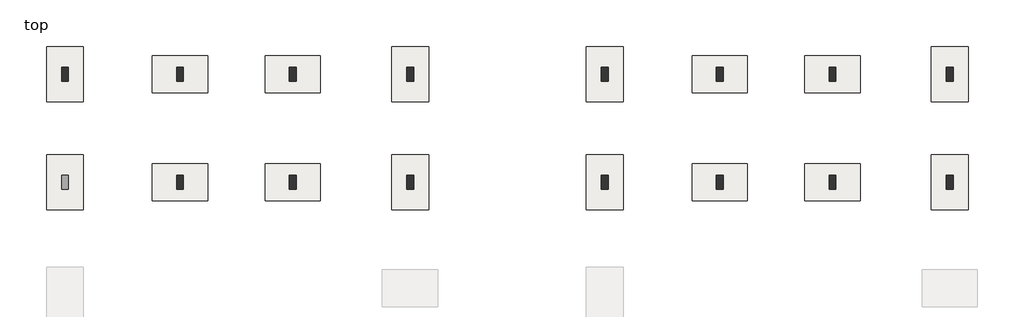
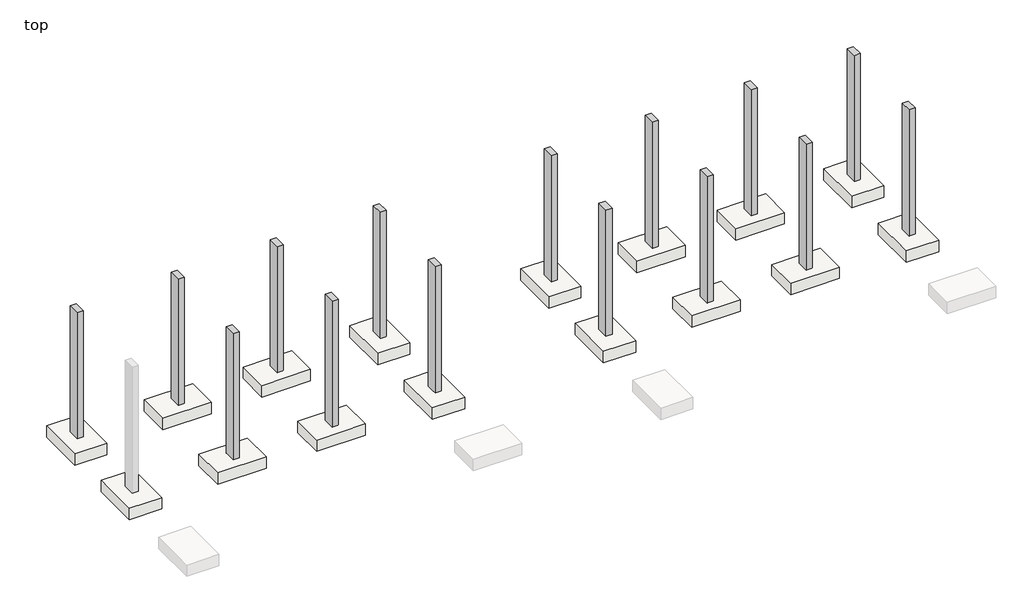
# One storey, part 2 of 2: 16 slabs, 15 columns.
"""IFC4 building model written with IfcOpenShell, lengths in millimetres."""

from ifc_helpers import new_model, si_unit, frame, origin, place, context, project, spatial, polyline, outline, extrude, faceted_brep, element, save

model = new_model("IFC4")

# Units and contexts
model_context = context("Model", 3, world=origin())
ifc_project = project(units=[si_unit("LENGTHUNIT", "METRE", prefix="MILLI")], contexts=[model_context])

# Site, building, storey
site = spatial("IfcSite", under=ifc_project)
building = spatial("IfcBuilding", under=site)
storey = spatial("IfcBuildingStorey", under=building, Name="top", Elevation=-1219.2)

# Columns
placement = place(None, origin())
element("IfcColumn", 1, ObjectType="Concrete-Rectangular-Column", at=placement, inside=storey, context=model_context, shape_type="Brep", body=[
    faceted_brep([(-16071.9993763, 6519.8935985, -1219.2), (-16071.9993763, 6062.6935985, -1219.2), (-16300.5993763, 6062.6935985, -1219.2), (-16300.5993763, 6519.8935985, -1219.2), (-16071.9993763, 6519.8935985, 3810.0), (-16071.9993763, 6062.6935985, 3810.0), (-16071.9993763, 6062.6935985, 609.6), (-16071.9993763, 6062.6935985, 0.0), (-16071.9993763, 6519.8935985, 0.0), (-16071.9993763, 6519.8935985, 609.6), (-16300.5993763, 6062.6935985, 3810.0), (-16300.5993763, 6062.6935985, 609.6), (-16300.5993763, 6062.6935985, 0.0), (-16300.5993763, 6519.8935985, 3810.0)], [[[0, 1, 2, 3]], [[4, 5, 6, 7, 1, 0, 8, 9]], [[5, 10, 11, 12, 2, 1, 7, 6]], [[10, 13, 3, 2, 12, 11]], [[13, 4, 9, 8, 0, 3]], [[4, 13, 10, 5]]]),
])
element("IfcColumn", 2, ObjectType="Concrete-Rectangular-Column", at=placement, inside=storey, context=model_context, shape_type="Brep", body=[
    faceted_brep([(-12261.9993763, 6519.8935985, -1219.2), (-12261.9993763, 6062.6935985, -1219.2), (-12490.5993763, 6062.6935985, -1219.2), (-12490.5993763, 6519.8935985, -1219.2), (-12261.9993763, 6519.8935985, 3810.0), (-12261.9993763, 6291.2935985, 3810.0), (-12261.9993763, 6062.6935985, 3810.0), (-12261.9993763, 6062.6935985, 609.6), (-12261.9993763, 6062.6935985, 0.0), (-12261.9993763, 6519.8935985, 0.0), (-12261.9993763, 6519.8935985, 609.6), (-12261.9993763, 6519.8935985, 3200.4), (-12490.5993763, 6062.6935985, 3810.0), (-12490.5993763, 6062.6935985, 609.6), (-12490.5993763, 6062.6935985, 0.0), (-12490.5993763, 6291.2935985, 3810.0), (-12490.5993763, 6519.8935985, 3810.0), (-12490.5993763, 6519.8935985, 3200.4), (-12490.5993763, 6519.8935985, 609.6), (-12490.5993763, 6519.8935985, 0.0)], [[[0, 1, 2, 3]], [[4, 5, 6, 7, 8, 1, 0, 9, 10, 11]], [[6, 12, 13, 14, 2, 1, 8, 7]], [[12, 15, 16, 17, 18, 19, 3, 2, 14, 13]], [[16, 4, 11, 10, 9, 0, 3, 19, 18, 17]], [[4, 16, 15, 12, 6, 5]]]),
])
element("IfcColumn", 3, ObjectType="Concrete-Rectangular-Column", at=placement, inside=storey, context=model_context, shape_type="Brep", body=[
    faceted_brep([(-8528.1993763, 6519.8935985, -1219.2), (-8528.1993763, 6062.6935985, -1219.2), (-8756.7993763, 6062.6935985, -1219.2), (-8756.7993763, 6519.8935985, -1219.2), (-8528.1993763, 6519.8935985, 3810.0), (-8528.1993763, 6291.2935985, 3810.0), (-8528.1993763, 6062.6935985, 3810.0), (-8528.1993763, 6062.6935985, 609.6), (-8528.1993763, 6062.6935985, 0.0), (-8528.1993763, 6519.8935985, 0.0), (-8528.1993763, 6519.8935985, 609.6), (-8528.1993763, 6519.8935985, 3200.4), (-8756.7993763, 6062.6935985, 3810.0), (-8756.7993763, 6062.6935985, 609.6), (-8756.7993763, 6062.6935985, 0.0), (-8756.7993763, 6291.2935985, 3810.0), (-8756.7993763, 6519.8935985, 3810.0), (-8756.7993763, 6519.8935985, 3200.4), (-8756.7993763, 6519.8935985, 609.6), (-8756.7993763, 6519.8935985, 0.0)], [[[0, 1, 2, 3]], [[4, 5, 6, 7, 8, 1, 0, 9, 10, 11]], [[6, 12, 13, 14, 2, 1, 8, 7]], [[12, 15, 16, 17, 18, 19, 3, 2, 14, 13]], [[16, 4, 11, 10, 9, 0, 3, 19, 18, 17]], [[4, 16, 15, 12, 6, 5]]]),
])
element("IfcColumn", 4, ObjectType="Concrete-Rectangular-Column", at=placement, inside=storey, context=model_context, shape_type="Brep", body=[
    faceted_brep([(-4641.9993763, 6519.8935985, -1219.2), (-4641.9993763, 6062.6935985, -1219.2), (-4870.5993763, 6062.6935985, -1219.2), (-4870.5993763, 6519.8935985, -1219.2), (-4641.9993763, 6519.8935985, 3810.0), (-4641.9993763, 6062.6935985, 3810.0), (-4641.9993763, 6062.6935985, 609.6), (-4641.9993763, 6062.6935985, 0.0), (-4870.5993763, 6062.6935985, 3810.0), (-4870.5993763, 6062.6935985, 609.6), (-4870.5993763, 6062.6935985, 0.0), (-4870.5993763, 6519.8935985, 3810.0), (-4870.5993763, 6519.8935985, 609.6), (-4870.5993763, 6519.8935985, 0.0)], [[[0, 1, 2, 3]], [[4, 5, 6, 7, 1, 0]], [[5, 8, 9, 10, 2, 1, 7, 6]], [[8, 11, 12, 13, 3, 2, 10, 9]], [[11, 4, 0, 3, 13, 12]], [[4, 11, 8, 5]]]),
])
element("IfcColumn", 5, ObjectType="Concrete-Rectangular-Column", at=placement, inside=storey, context=model_context, shape_type="Brep", body=[
    faceted_brep([(-12261.9993763, 2938.4935985, -1219.2), (-12261.9993763, 2481.2935985, -1219.2), (-12490.5993763, 2481.2935985, -1219.2), (-12490.5993763, 2938.4935985, -1219.2), (-12261.9993763, 2938.4935985, 3810.0), (-12261.9993763, 2772.356095, 3810.0), (-12261.9993763, 2709.8935985, 3810.0), (-12261.9993763, 2481.2935985, 3810.0), (-12261.9993763, 2481.2935985, 3200.4), (-12261.9993763, 2481.2935985, 609.6), (-12261.9993763, 2481.2935985, 0.0), (-12261.9993763, 2938.4935985, 0.0), (-12261.9993763, 2938.4935985, 609.6), (-12261.9993763, 2938.4935985, 3200.4), (-12490.5993763, 2481.2935985, 3810.0), (-12490.5993763, 2481.2935985, 3200.4), (-12490.5993763, 2481.2935985, 609.6), (-12490.5993763, 2481.2935985, 0.0), (-12490.5993763, 2546.6730431, 3810.0), (-12490.5993763, 2775.2918938, 3810.0), (-12490.5993763, 2938.4935985, 3810.0), (-12490.5993763, 2938.4935985, 3200.4), (-12490.5993763, 2938.4935985, 609.6), (-12490.5993763, 2938.4935985, 0.0)], [[[0, 1, 2, 3]], [[4, 5, 6, 7, 8, 9, 10, 1, 0, 11, 12, 13]], [[7, 14, 15, 16, 17, 2, 1, 10, 9, 8]], [[14, 18, 19, 20, 21, 22, 23, 3, 2, 17, 16, 15]], [[20, 4, 13, 12, 11, 0, 3, 23, 22, 21]], [[4, 20, 19, 18, 14, 7, 6, 5]]]),
])
element("IfcColumn", 6, ObjectType="Concrete-Rectangular-Column", at=placement, inside=storey, context=model_context, shape_type="Brep", body=[
    faceted_brep([(-4641.9993763, 2938.4935985, -1219.2), (-4641.9993763, 2481.2935985, -1219.2), (-4870.5993763, 2481.2935985, -1219.2), (-4870.5993763, 2938.4935985, -1219.2), (-4641.9993763, 2938.4935985, 3810.0), (-4641.9993763, 2481.2935985, 3810.0), (-4641.9993763, 2481.2935985, 3200.4), (-4641.9993763, 2481.2935985, 609.6), (-4641.9993763, 2481.2935985, 0.0), (-4641.9993763, 2938.4935985, 0.0), (-4641.9993763, 2938.4935985, 609.6), (-4641.9993763, 2938.4935985, 3200.4), (-4870.5993763, 2481.2935985, 3810.0), (-4870.5993763, 2481.2935985, 3200.4), (-4870.5993763, 2481.2935985, 609.6), (-4870.5993763, 2481.2935985, 0.0), (-4870.5993763, 2938.4935985, 3810.0), (-4870.5993763, 2938.4935985, 3200.4), (-4870.5993763, 2938.4935985, 609.6), (-4870.5993763, 2938.4935985, 0.0)], [[[0, 1, 2, 3]], [[4, 5, 6, 7, 8, 1, 0, 9, 10, 11]], [[5, 12, 13, 14, 15, 2, 1, 8, 7, 6]], [[12, 16, 17, 18, 19, 3, 2, 15, 14, 13]], [[16, 4, 11, 10, 9, 0, 3, 19, 18, 17]], [[4, 16, 12, 5]]]),
])
element("IfcColumn", 7, ObjectType="Concrete-Rectangular-Column", at=placement, inside=storey, context=model_context, shape_type="Brep", body=[
    faceted_brep([(-8528.1993763, 2938.4935985, -1219.2), (-8528.1993763, 2481.2935985, -1219.2), (-8756.7993763, 2481.2935985, -1219.2), (-8756.7993763, 2938.4935985, -1219.2), (-8528.1993763, 2938.4935985, 3810.0), (-8528.1993763, 2724.4047146, 3810.0), (-8528.1993763, 2709.8935985, 3810.0), (-8528.1993763, 2481.2935985, 3810.0), (-8528.1993763, 2481.2935985, 3200.4), (-8528.1993763, 2481.2935985, 609.6), (-8528.1993763, 2481.2935985, 0.0), (-8528.1993763, 2938.4935985, 0.0), (-8528.1993763, 2938.4935985, 609.6), (-8528.1993763, 2938.4935985, 3200.4), (-8756.7993763, 2481.2935985, 3810.0), (-8756.7993763, 2481.2935985, 3200.4), (-8756.7993763, 2481.2935985, 609.6), (-8756.7993763, 2481.2935985, 0.0), (-8756.7993763, 2709.8935985, 3810.0), (-8756.7993763, 2727.3405134, 3810.0), (-8756.7993763, 2938.4935985, 3810.0), (-8756.7993763, 2938.4935985, 3200.4), (-8756.7993763, 2938.4935985, 609.6), (-8756.7993763, 2938.4935985, 0.0)], [[[0, 1, 2, 3]], [[4, 5, 6, 7, 8, 9, 10, 1, 0, 11, 12, 13]], [[7, 14, 15, 16, 17, 2, 1, 10, 9, 8]], [[14, 18, 19, 20, 21, 22, 23, 3, 2, 17, 16, 15]], [[20, 4, 13, 12, 11, 0, 3, 23, 22, 21]], [[4, 20, 19, 18, 14, 7, 6, 5]]]),
])
element("IfcColumn", 8, ObjectType="Concrete-Rectangular-Column", at=placement, inside=storey, context=model_context, shape_type="Brep", body=[
    faceted_brep([(1802.5761273, 6519.8935985, -1219.2), (1802.5761273, 6062.6935985, -1219.2), (1573.9761273, 6062.6935985, -1219.2), (1573.9761273, 6519.8935985, -1219.2), (1802.5761273, 6519.8935985, 3810.0), (1802.5761273, 6062.6935985, 3810.0), (1802.5761273, 6062.6935985, 609.6), (1802.5761273, 6062.6935985, 0.0), (1802.5761273, 6519.8935985, 0.0), (1802.5761273, 6519.8935985, 609.6), (1573.9761273, 6062.6935985, 3810.0), (1573.9761273, 6062.6935985, 609.6), (1573.9761273, 6062.6935985, 0.0), (1573.9761273, 6519.8935985, 3810.0)], [[[0, 1, 2, 3]], [[4, 5, 6, 7, 1, 0, 8, 9]], [[5, 10, 11, 12, 2, 1, 7, 6]], [[10, 13, 3, 2, 12, 11]], [[13, 4, 9, 8, 0, 3]], [[4, 13, 10, 5]]]),
])
element("IfcColumn", 9, ObjectType="Concrete-Rectangular-Column", at=placement, inside=storey, context=model_context, shape_type="Brep", body=[
    faceted_brep([(5612.5761273, 6519.8935985, -1219.2), (5612.5761273, 6062.6935985, -1219.2), (5383.9761273, 6062.6935985, -1219.2), (5383.9761273, 6519.8935985, -1219.2), (5612.5761273, 6519.8935985, 3810.0), (5612.5761273, 6291.2935985, 3810.0), (5612.5761273, 6062.6935985, 3810.0), (5612.5761273, 6062.6935985, 609.6), (5612.5761273, 6062.6935985, 0.0), (5612.5761273, 6519.8935985, 0.0), (5612.5761273, 6519.8935985, 609.6), (5612.5761273, 6519.8935985, 3200.4), (5383.9761273, 6062.6935985, 3810.0), (5383.9761273, 6062.6935985, 609.6), (5383.9761273, 6062.6935985, 0.0), (5383.9761273, 6291.2935985, 3810.0), (5383.9761273, 6519.8935985, 3810.0), (5383.9761273, 6519.8935985, 3200.4), (5383.9761273, 6519.8935985, 609.6), (5383.9761273, 6519.8935985, 0.0)], [[[0, 1, 2, 3]], [[4, 5, 6, 7, 8, 1, 0, 9, 10, 11]], [[6, 12, 13, 14, 2, 1, 8, 7]], [[12, 15, 16, 17, 18, 19, 3, 2, 14, 13]], [[16, 4, 11, 10, 9, 0, 3, 19, 18, 17]], [[4, 16, 15, 12, 6, 5]]]),
])
element("IfcColumn", 10, ObjectType="Concrete-Rectangular-Column", at=placement, inside=storey, context=model_context, shape_type="Brep", body=[
    faceted_brep([(9346.3761273, 6519.8935985, -1219.2), (9346.3761273, 6062.6935985, -1219.2), (9117.7761273, 6062.6935985, -1219.2), (9117.7761273, 6519.8935985, -1219.2), (9346.3761273, 6519.8935985, 3810.0), (9346.3761273, 6291.2935985, 3810.0), (9346.3761273, 6062.6935985, 3810.0), (9346.3761273, 6062.6935985, 609.6), (9346.3761273, 6062.6935985, 0.0), (9346.3761273, 6519.8935985, 0.0), (9346.3761273, 6519.8935985, 609.6), (9346.3761273, 6519.8935985, 3200.4), (9117.7761273, 6062.6935985, 3810.0), (9117.7761273, 6062.6935985, 609.6), (9117.7761273, 6062.6935985, 0.0), (9117.7761273, 6291.2935985, 3810.0), (9117.7761273, 6519.8935985, 3810.0), (9117.7761273, 6519.8935985, 3200.4), (9117.7761273, 6519.8935985, 609.6), (9117.7761273, 6519.8935985, 0.0)], [[[0, 1, 2, 3]], [[4, 5, 6, 7, 8, 1, 0, 9, 10, 11]], [[6, 12, 13, 14, 2, 1, 8, 7]], [[12, 15, 16, 17, 18, 19, 3, 2, 14, 13]], [[16, 4, 11, 10, 9, 0, 3, 19, 18, 17]], [[4, 16, 15, 12, 6, 5]]]),
])
element("IfcColumn", 11, ObjectType="Concrete-Rectangular-Column", at=placement, inside=storey, context=model_context, shape_type="Brep", body=[
    faceted_brep([(13232.5761273, 6519.8935985, -1219.2), (13232.5761273, 6062.6935985, -1219.2), (13003.9761273, 6062.6935985, -1219.2), (13003.9761273, 6519.8935985, -1219.2), (13232.5761273, 6519.8935985, 3810.0), (13232.5761273, 6062.6935985, 3810.0), (13232.5761273, 6062.6935985, 609.6), (13232.5761273, 6062.6935985, 0.0), (13003.9761273, 6062.6935985, 3810.0), (13003.9761273, 6062.6935985, 609.6), (13003.9761273, 6062.6935985, 0.0), (13003.9761273, 6519.8935985, 3810.0), (13003.9761273, 6519.8935985, 609.6), (13003.9761273, 6519.8935985, 0.0)], [[[0, 1, 2, 3]], [[4, 5, 6, 7, 1, 0]], [[5, 8, 9, 10, 2, 1, 7, 6]], [[8, 11, 12, 13, 3, 2, 10, 9]], [[11, 4, 0, 3, 13, 12]], [[4, 11, 8, 5]]]),
])
element("IfcColumn", 12, ObjectType="Concrete-Rectangular-Column", at=placement, inside=storey, context=model_context, shape_type="Brep", body=[
    faceted_brep([(5612.5761273, 2938.4935985, -1219.2), (5612.5761273, 2481.2935985, -1219.2), (5383.9761273, 2481.2935985, -1219.2), (5383.9761273, 2938.4935985, -1219.2), (5612.5761273, 2938.4935985, 3810.0), (5612.5761273, 2772.356095, 3810.0), (5612.5761273, 2543.7372443, 3810.0), (5612.5761273, 2481.2935985, 3810.0), (5612.5761273, 2481.2935985, 3200.4), (5612.5761273, 2481.2935985, 609.6), (5612.5761273, 2481.2935985, 0.0), (5612.5761273, 2938.4935985, 0.0), (5612.5761273, 2938.4935985, 609.6), (5612.5761273, 2938.4935985, 3200.4), (5383.9761273, 2481.2935985, 3810.0), (5383.9761273, 2481.2935985, 3200.4), (5383.9761273, 2481.2935985, 609.6), (5383.9761273, 2481.2935985, 0.0), (5383.9761273, 2546.6730431, 3810.0), (5383.9761273, 2775.2918938, 3810.0), (5383.9761273, 2938.4935985, 3810.0), (5383.9761273, 2938.4935985, 3200.4), (5383.9761273, 2938.4935985, 609.6), (5383.9761273, 2938.4935985, 0.0)], [[[0, 1, 2, 3]], [[4, 5, 6, 7, 8, 9, 10, 1, 0, 11, 12, 13]], [[7, 14, 15, 16, 17, 2, 1, 10, 9, 8]], [[14, 18, 19, 20, 21, 22, 23, 3, 2, 17, 16, 15]], [[20, 4, 13, 12, 11, 0, 3, 23, 22, 21]], [[4, 20, 19, 18, 14, 7, 6, 5]]]),
])
element("IfcColumn", 13, ObjectType="Concrete-Rectangular-Column", at=placement, inside=storey, context=model_context, shape_type="Brep", body=[
    faceted_brep([(1802.5761273, 2938.4935985, -1219.2), (1802.5761273, 2481.2935985, -1219.2), (1573.9761273, 2481.2935985, -1219.2), (1573.9761273, 2938.4935985, -1219.2), (1802.5761273, 2938.4935985, 3810.0), (1802.5761273, 2481.2935985, 3810.0), (1802.5761273, 2481.2935985, 3200.4), (1802.5761273, 2481.2935985, 609.6), (1802.5761273, 2481.2935985, 0.0), (1802.5761273, 2938.4935985, 0.0), (1802.5761273, 2938.4935985, 609.6), (1802.5761273, 2938.4935985, 3200.4), (1573.9761273, 2481.2935985, 3810.0), (1573.9761273, 2481.2935985, 3200.4), (1573.9761273, 2481.2935985, 609.6), (1573.9761273, 2481.2935985, 0.0), (1573.9761273, 2938.4935985, 3810.0), (1573.9761273, 2938.4935985, 3200.4), (1573.9761273, 2938.4935985, 609.6), (1573.9761273, 2938.4935985, 0.0)], [[[0, 1, 2, 3]], [[4, 5, 6, 7, 8, 1, 0, 9, 10, 11]], [[5, 12, 13, 14, 15, 2, 1, 8, 7, 6]], [[12, 16, 17, 18, 19, 3, 2, 15, 14, 13]], [[16, 4, 11, 10, 9, 0, 3, 19, 18, 17]], [[4, 16, 12, 5]]]),
])
element("IfcColumn", 14, ObjectType="Concrete-Rectangular-Column", at=placement, inside=storey, context=model_context, shape_type="Brep", body=[
    faceted_brep([(13232.5761273, 2938.4935985, -1219.2), (13232.5761273, 2481.2935985, -1219.2), (13003.9761273, 2481.2935985, -1219.2), (13003.9761273, 2938.4935985, -1219.2), (13232.5761273, 2938.4935985, 3810.0), (13232.5761273, 2481.2935985, 3810.0), (13232.5761273, 2481.2935985, 3200.4), (13232.5761273, 2481.2935985, 609.6), (13232.5761273, 2481.2935985, 0.0), (13232.5761273, 2938.4935985, 0.0), (13232.5761273, 2938.4935985, 609.6), (13232.5761273, 2938.4935985, 3200.4), (13003.9761273, 2481.2935985, 3810.0), (13003.9761273, 2481.2935985, 3200.4), (13003.9761273, 2481.2935985, 609.6), (13003.9761273, 2481.2935985, 0.0), (13003.9761273, 2938.4935985, 3810.0), (13003.9761273, 2938.4935985, 3200.4), (13003.9761273, 2938.4935985, 609.6), (13003.9761273, 2938.4935985, 0.0)], [[[0, 1, 2, 3]], [[4, 5, 6, 7, 8, 1, 0, 9, 10, 11]], [[5, 12, 13, 14, 15, 2, 1, 8, 7, 6]], [[12, 16, 17, 18, 19, 3, 2, 15, 14, 13]], [[16, 4, 11, 10, 9, 0, 3, 19, 18, 17]], [[4, 16, 12, 5]]]),
])
element("IfcColumn", 15, ObjectType="Concrete-Rectangular-Column", at=placement, inside=storey, context=model_context, shape_type="Brep", body=[
    faceted_brep([(9346.3761273, 2938.4935985, -1219.2), (9346.3761273, 2481.2935985, -1219.2), (9117.7761273, 2481.2935985, -1219.2), (9117.7761273, 2938.4935985, -1219.2), (9346.3761273, 2938.4935985, 3810.0), (9346.3761273, 2724.4047146, 3810.0), (9346.3761273, 2709.8935985, 3810.0), (9346.3761273, 2495.7858639, 3810.0), (9346.3761273, 2481.2935985, 3810.0), (9346.3761273, 2481.2935985, 3200.4), (9346.3761273, 2481.2935985, 609.6), (9346.3761273, 2481.2935985, 0.0), (9346.3761273, 2938.4935985, 0.0), (9346.3761273, 2938.4935985, 609.6), (9346.3761273, 2938.4935985, 3200.4), (9117.7761273, 2481.2935985, 3810.0), (9117.7761273, 2481.2935985, 3200.4), (9117.7761273, 2481.2935985, 609.6), (9117.7761273, 2481.2935985, 0.0), (9117.7761273, 2498.7216627, 3810.0), (9117.7761273, 2709.8935985, 3810.0), (9117.7761273, 2727.3405134, 3810.0), (9117.7761273, 2938.4935985, 3810.0), (9117.7761273, 2938.4935985, 3200.4), (9117.7761273, 2938.4935985, 609.6), (9117.7761273, 2938.4935985, 0.0)], [[[0, 1, 2, 3]], [[4, 5, 6, 7, 8, 9, 10, 11, 1, 0, 12, 13, 14]], [[8, 15, 16, 17, 18, 2, 1, 11, 10, 9]], [[15, 19, 20, 21, 22, 23, 24, 25, 3, 2, 18, 17, 16]], [[22, 4, 14, 13, 12, 0, 3, 25, 24, 23]], [[4, 22, 21, 20, 19, 15, 8, 7, 6, 5]]]),
])

# Slabs
element("IfcSlab", 16, ObjectType="Footing-Rectangular : 72\" x 48\" x 18\"", at=placement, inside=storey, context=model_context, shape_type="SweptSolid", body=[
    extrude(outline(polyline([(-15576.6993763, 7205.6935985), (-15576.6993763, 5376.8935985), (-16795.8993763, 5376.8935985), (-16795.8993763, 7205.6935985), (-15576.6993763, 7205.6935985)])), frame((0.0, 0.0, -1676.4), z_axis=(0.0, 0.0, 1.0), x_axis=(1.0, 0.0, 0.0)), (0.0, 0.0, 1.0), 457.2),
])
element("IfcSlab", 17, ObjectType="Footing-Rectangular : 72\" x 48\" x 18\"", at=placement, inside=storey, context=model_context, shape_type="SweptSolid", body=[
    extrude(outline(polyline([(-13290.6993763, 6900.8935985), (-11461.8993763, 6900.8935985), (-11461.8993763, 5681.6935985), (-13290.6993763, 5681.6935985), (-13290.6993763, 6900.8935985)])), frame((0.0, 0.0, -1676.4), z_axis=(0.0, 0.0, 1.0), x_axis=(1.0, 0.0, 0.0)), (0.0, 0.0, 1.0), 457.2),
])
element("IfcSlab", 18, ObjectType="Footing-Rectangular : 72\" x 48\" x 18\"", at=placement, inside=storey, context=model_context, shape_type="SweptSolid", body=[
    extrude(outline(polyline([(-9556.8993763, 6900.8935985), (-7728.0993763, 6900.8935985), (-7728.0993763, 5681.6935985), (-9556.8993763, 5681.6935985), (-9556.8993763, 6900.8935985)])), frame((0.0, 0.0, -1676.4), z_axis=(0.0, 0.0, 1.0), x_axis=(1.0, 0.0, 0.0)), (0.0, 0.0, 1.0), 457.2),
])
element("IfcSlab", 19, ObjectType="Footing-Rectangular : 72\" x 48\" x 18\"", at=placement, inside=storey, context=model_context, shape_type="SweptSolid", body=[
    extrude(outline(polyline([(-4146.6993763, 7205.6935985), (-4146.6993763, 5376.8935985), (-5365.8993763, 5376.8935985), (-5365.8993763, 7205.6935985), (-4146.6993763, 7205.6935985)])), frame((0.0, 0.0, -1676.4), z_axis=(0.0, 0.0, 1.0), x_axis=(1.0, 0.0, 0.0)), (0.0, 0.0, 1.0), 457.2),
])
element("IfcSlab", 20, ObjectType="Footing-Rectangular : 72\" x 48\" x 18\"", at=placement, inside=storey, context=model_context, shape_type="SweptSolid", body=[
    extrude(outline(polyline([(-13290.6993763, 3319.4935985), (-11461.8993763, 3319.4935985), (-11461.8993763, 2100.2935985), (-13290.6993763, 2100.2935985), (-13290.6993763, 3319.4935985)])), frame((0.0, 0.0, -1676.4), z_axis=(0.0, 0.0, 1.0), x_axis=(1.0, 0.0, 0.0)), (0.0, 0.0, 1.0), 457.2),
])
element("IfcSlab", 21, ObjectType="Footing-Rectangular : 72\" x 48\" x 18\"", at=placement, inside=storey, context=model_context, shape_type="SweptSolid", body=[
    extrude(outline(polyline([(-15576.6993763, 3624.2935985), (-15576.6993763, 1795.4935985), (-16795.8993763, 1795.4935985), (-16795.8993763, 3624.2935985), (-15576.6993763, 3624.2935985)])), frame((0.0, 0.0, -1676.4), z_axis=(0.0, 0.0, 1.0), x_axis=(1.0, 0.0, 0.0)), (0.0, 0.0, 1.0), 457.2),
])
element("IfcSlab", 22, ObjectType="Footing-Rectangular : 72\" x 48\" x 18\"", at=placement, inside=storey, context=model_context, shape_type="SweptSolid", body=[
    extrude(outline(polyline([(-4146.6993763, 3624.2935985), (-4146.6993763, 1795.4935985), (-5365.8993763, 1795.4935985), (-5365.8993763, 3624.2935985), (-4146.6993763, 3624.2935985)])), frame((0.0, 0.0, -1676.4), z_axis=(0.0, 0.0, 1.0), x_axis=(1.0, 0.0, 0.0)), (0.0, 0.0, 1.0), 457.2),
])
element("IfcSlab", 23, ObjectType="Footing-Rectangular : 72\" x 48\" x 18\"", at=placement, inside=storey, context=model_context, shape_type="SweptSolid", body=[
    extrude(outline(polyline([(-9556.8993763, 3319.4935985), (-7728.0993763, 3319.4935985), (-7728.0993763, 2100.2935985), (-9556.8993763, 2100.2935985), (-9556.8993763, 3319.4935985)])), frame((0.0, 0.0, -1676.4), z_axis=(0.0, 0.0, 1.0), x_axis=(1.0, 0.0, 0.0)), (0.0, 0.0, 1.0), 457.2),
])
element("IfcSlab", 24, ObjectType="Footing-Rectangular : 72\" x 48\" x 18\"", at=placement, inside=storey, context=model_context, shape_type="SweptSolid", body=[
    extrude(outline(polyline([(2297.8761273, 7205.6935985), (2297.8761273, 5376.8935985), (1078.6761273, 5376.8935985), (1078.6761273, 7205.6935985), (2297.8761273, 7205.6935985)])), frame((0.0, 0.0, -1676.4), z_axis=(0.0, 0.0, 1.0), x_axis=(1.0, 0.0, 0.0)), (0.0, 0.0, 1.0), 457.2),
])
element("IfcSlab", 25, ObjectType="Footing-Rectangular : 72\" x 48\" x 18\"", at=placement, inside=storey, context=model_context, shape_type="SweptSolid", body=[
    extrude(outline(polyline([(4583.8761273, 6900.8935985), (6412.6761273, 6900.8935985), (6412.6761273, 5681.6935985), (4583.8761273, 5681.6935985), (4583.8761273, 6900.8935985)])), frame((0.0, 0.0, -1676.4), z_axis=(0.0, 0.0, 1.0), x_axis=(1.0, 0.0, 0.0)), (0.0, 0.0, 1.0), 457.2),
])
element("IfcSlab", 26, ObjectType="Footing-Rectangular : 72\" x 48\" x 18\"", at=placement, inside=storey, context=model_context, shape_type="SweptSolid", body=[
    extrude(outline(polyline([(8317.6761273, 6900.8935985), (10146.4761273, 6900.8935985), (10146.4761273, 5681.6935985), (8317.6761273, 5681.6935985), (8317.6761273, 6900.8935985)])), frame((0.0, 0.0, -1676.4), z_axis=(0.0, 0.0, 1.0), x_axis=(1.0, 0.0, 0.0)), (0.0, 0.0, 1.0), 457.2),
])
element("IfcSlab", 27, ObjectType="Footing-Rectangular : 72\" x 48\" x 18\"", at=placement, inside=storey, context=model_context, shape_type="SweptSolid", body=[
    extrude(outline(polyline([(13727.8761273, 7205.6935985), (13727.8761273, 5376.8935985), (12508.6761273, 5376.8935985), (12508.6761273, 7205.6935985), (13727.8761273, 7205.6935985)])), frame((0.0, 0.0, -1676.4), z_axis=(0.0, 0.0, 1.0), x_axis=(1.0, 0.0, 0.0)), (0.0, 0.0, 1.0), 457.2),
])
element("IfcSlab", 28, ObjectType="Footing-Rectangular : 72\" x 48\" x 18\"", at=placement, inside=storey, context=model_context, shape_type="SweptSolid", body=[
    extrude(outline(polyline([(4583.8761273, 3319.4935985), (6412.6761273, 3319.4935985), (6412.6761273, 2100.2935985), (4583.8761273, 2100.2935985), (4583.8761273, 3319.4935985)])), frame((0.0, 0.0, -1676.4), z_axis=(0.0, 0.0, 1.0), x_axis=(1.0, 0.0, 0.0)), (0.0, 0.0, 1.0), 457.2),
])
element("IfcSlab", 29, ObjectType="Footing-Rectangular : 72\" x 48\" x 18\"", at=placement, inside=storey, context=model_context, shape_type="SweptSolid", body=[
    extrude(outline(polyline([(2297.8761273, 3624.2935985), (2297.8761273, 1795.4935985), (1078.6761273, 1795.4935985), (1078.6761273, 3624.2935985), (2297.8761273, 3624.2935985)])), frame((0.0, 0.0, -1676.4), z_axis=(0.0, 0.0, 1.0), x_axis=(1.0, 0.0, 0.0)), (0.0, 0.0, 1.0), 457.2),
])
element("IfcSlab", 30, ObjectType="Footing-Rectangular : 72\" x 48\" x 18\"", at=placement, inside=storey, context=model_context, shape_type="SweptSolid", body=[
    extrude(outline(polyline([(13727.8761273, 3624.2935985), (13727.8761273, 1795.4935985), (12508.6761273, 1795.4935985), (12508.6761273, 3624.2935985), (13727.8761273, 3624.2935985)])), frame((0.0, 0.0, -1676.4), z_axis=(0.0, 0.0, 1.0), x_axis=(1.0, 0.0, 0.0)), (0.0, 0.0, 1.0), 457.2),
])
element("IfcSlab", 31, ObjectType="Footing-Rectangular : 72\" x 48\" x 18\"", at=placement, inside=storey, context=model_context, shape_type="SweptSolid", body=[
    extrude(outline(polyline([(8317.6761273, 3319.4935985), (10146.4761273, 3319.4935985), (10146.4761273, 2100.2935985), (8317.6761273, 2100.2935985), (8317.6761273, 3319.4935985)])), frame((0.0, 0.0, -1676.4), z_axis=(0.0, 0.0, 1.0), x_axis=(1.0, 0.0, 0.0)), (0.0, 0.0, 1.0), 457.2),
])

save(model, "model.ifc")

# Revit data of these elements
# Type "Concrete-Rectangular-Column"
#   Assembly Code = "B10"
#   b = 0' - 9"
#   h = 1' - 6"
#   Structural Material [instance default] = Concrete, Cast-in-Place gray
# Type "Footing-Rectangular : 72\" x 48\" x 18\""
#   Assembly Code = "A1010100"
#   Width = 4' - 0"
#   Length = 6' - 0"
#   Foundation Thickness = 1' - 6"
#   Structural Material [instance default] = Concrete, Cast-in-Place gray
# Elements 1, 2, 3, 4, 5, 6, 7, 8, 9, 10, 11, 12, 13, 14, 15 (IfcColumn, "Concrete-Rectangular-Column")
#   Structural Material = Concrete, Cast-in-Place gray
#   Phase Created = New Construction
#   Materials on its faces: "Concrete, Cast-in-Place gray"
# Elements 16, 17, 18, 19, 20, 21, 22, 23, 24, 25, 26, 27, 28, 29, 30, 31 (IfcSlab, "Footing-Rectangular : 72\" x 48\" x 18\"")
#   Structural Material = Concrete, Cast-in-Place gray
#   Phase Created = New Construction
#   Materials on its faces: "Concrete, Cast-in-Place gray"
# Materials
#   "Concrete, Cast-in-Place gray": class "Concrete", colour RGB 192 192 192, transparency 0, Description = "Cast-in-place concrete", Cost = 0
